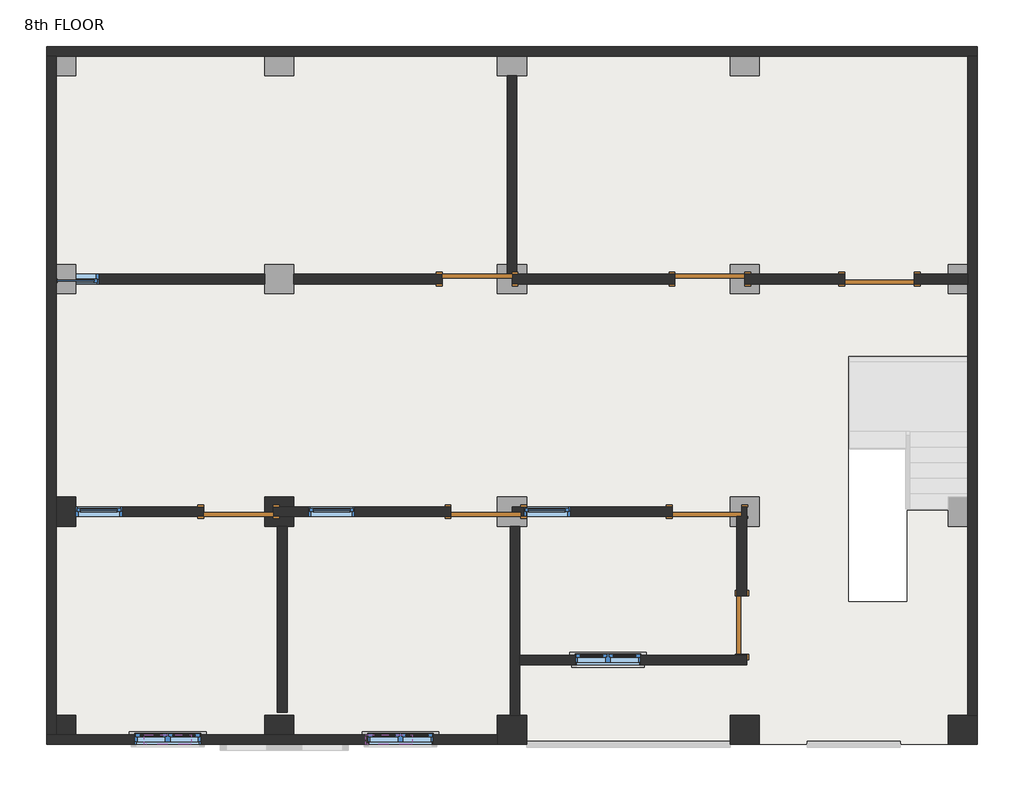
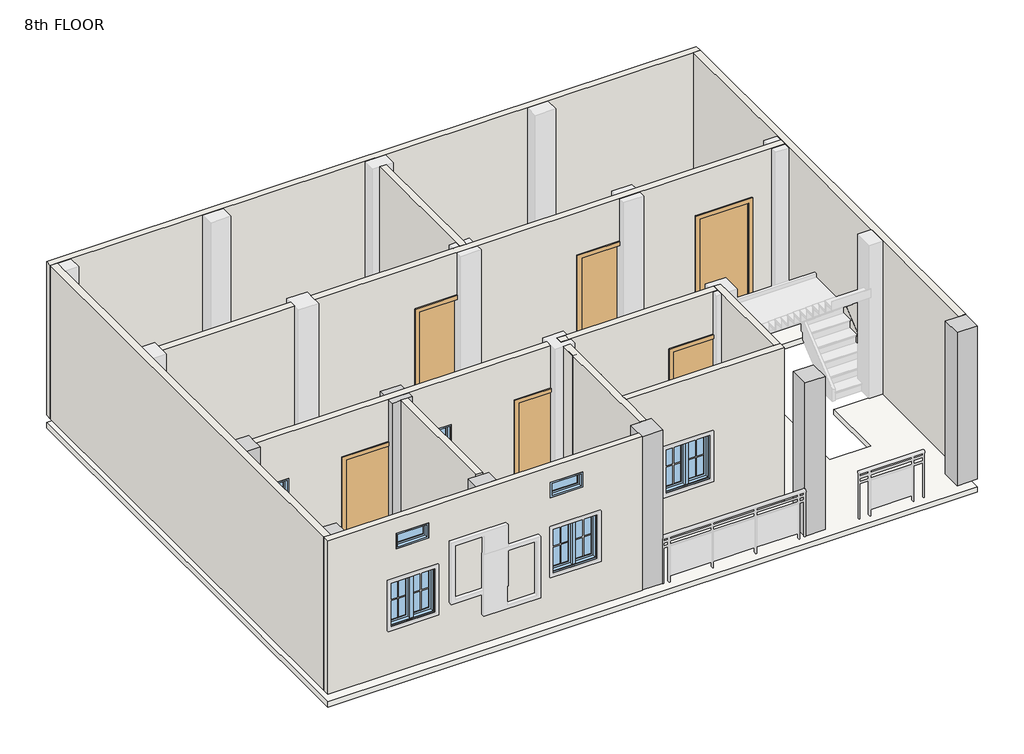
# One storey, part 1 of 2: 15 walls, 9 windows, 7 columns, 7 doors, 1 slab.
"""IFC4 building model written with IfcOpenShell, lengths in millimetres."""

from ifc_helpers import new_model, si_unit, frame, origin, place, context, project, spatial, polyline, outline, extrude, faceted_brep, transform, mapped, element, save
from components import door_e00f436c, door_a1797ceb, window_4c2727af, window_0bf3737e, window_78893e6c, window_0d9958e7

model = new_model("IFC4")

# Units and contexts
model_context = context("Model", 3, world=origin())
ifc_project = project(units=[si_unit("LENGTHUNIT", "METRE", prefix="MILLI")], contexts=[model_context])

# Site, building, storey
site = spatial("IfcSite", under=ifc_project)
building = spatial("IfcBuilding", under=site)
storey = spatial("IfcBuildingStorey", under=building, Name="8th FLOOR", Elevation=24231.6)

# Columns
placement = place(None, origin())
element("IfcColumn", 1, ObjectType="column family : column family", at=placement, inside=storey, context=model_context, shape_type="Brep", body=[
    faceted_brep([(-12576.097125, 2486.2065522, 24236.6), (-12957.097125, 2486.2065522, 24236.6), (-12957.097125, 2867.2065522, 24236.6), (-12576.097125, 2867.2065522, 24236.6), (-12576.097125, 2740.2065522, 24236.6), (-12842.797125, 2740.2065522, 24236.6), (-12842.797125, 2613.2065522, 24236.6), (-12576.097125, 2613.2065522, 24236.6), (-12576.097125, 2486.2065522, 27274.6), (-12576.097125, 2613.2065522, 27274.6), (-12957.097125, 2486.2065522, 27274.6), (-12957.097125, 2613.2065522, 27274.6), (-12957.097125, 2613.2065522, 26365.2), (-12957.097125, 2740.2065522, 26365.2), (-12957.097125, 2740.2065522, 27274.6), (-12957.097125, 2867.2065522, 27274.6), (-12576.097125, 2867.2065522, 27274.6), (-12842.797125, 2613.2065522, 26365.2), (-12842.797125, 2740.2065522, 26365.2), (-12576.097125, 2740.2065522, 27274.6)], [[[0, 1, 2, 3, 4, 5, 6, 7]], [[8, 0, 7, 9]], [[1, 0, 8, 10]], [[2, 1, 10, 11, 12, 13, 14, 15]], [[3, 2, 15, 16]], [[10, 8, 9, 11]], [[6, 17, 12, 11, 9, 7]], [[13, 18, 5, 4, 19, 14]], [[3, 16, 19, 4]], [[16, 15, 14, 19]], [[17, 18, 13, 12]], [[18, 17, 6, 5]]]),
])
element("IfcColumn", 2, ObjectType="column family : column family", at=placement, inside=storey, context=model_context, shape_type="SweptSolid", body=[
    extrude(outline(polyline([(-15433.597125, 2867.2065522), (-15433.597125, 2486.2065522), (-15687.597125, 2486.2065522), (-15687.597125, 2867.2065522), (-15433.597125, 2867.2065522)])), frame((0.0, 0.0, 24236.6), z_axis=(0.0, 0.0, 1.0), x_axis=(1.0, 0.0, 0.0)), (0.0, 0.0, 1.0), 3038.0),
])
element("IfcColumn", 3, ObjectType="column family : column family", at=placement, inside=storey, context=model_context, shape_type="SweptSolid", body=[
    extrude(outline(polyline([(-15433.597125, 9.7065522), (-15433.597125, -244.2934478), (-15687.597125, -244.2934478), (-15687.597125, 9.7065522), (-15433.597125, 9.7065522)])), frame((0.0, 0.0, 24236.6), z_axis=(0.0, 0.0, 1.0), x_axis=(1.0, 0.0, 0.0)), (0.0, 0.0, 1.0), 3038.0),
])
element("IfcColumn", 4, ObjectType="column family : column family", at=placement, inside=storey, context=model_context, shape_type="SweptSolid", body=[
    extrude(outline(polyline([(-3622.597125, 9.7065522), (-3622.597125, -371.2934478), (-4003.597125, -371.2934478), (-4003.597125, 9.7065522), (-3622.597125, 9.7065522)])), frame((0.0, 0.0, 24236.6), z_axis=(0.0, 0.0, 1.0), x_axis=(1.0, 0.0, 0.0)), (0.0, 0.0, 1.0), 3038.0),
])
element("IfcColumn", 5, ObjectType="column family : column family", at=placement, inside=storey, context=model_context, shape_type="SweptSolid", body=[
    extrude(outline(polyline([(-6480.097125, 9.7065522), (-6480.097125, -371.2934478), (-6861.097125, -371.2934478), (-6861.097125, 9.7065522), (-6480.097125, 9.7065522)])), frame((0.0, 0.0, 24236.6), z_axis=(0.0, 0.0, 1.0), x_axis=(1.0, 0.0, 0.0)), (0.0, 0.0, 1.0), 3038.0),
])
element("IfcColumn", 6, ObjectType="column family : column family", at=placement, inside=storey, context=model_context, shape_type="SweptSolid", body=[
    extrude(outline(polyline([(-9528.097125, 9.7065522), (-9528.097125, -371.2934478), (-9909.097125, -371.2934478), (-9909.097125, 9.7065522), (-9528.097125, 9.7065522)])), frame((0.0, 0.0, 24236.6), z_axis=(0.0, 0.0, 1.0), x_axis=(1.0, 0.0, 0.0)), (0.0, 0.0, 1.0), 3038.0),
])
element("IfcColumn", 7, ObjectType="column family : column family", at=placement, inside=storey, context=model_context, shape_type="SweptSolid", body=[
    extrude(outline(polyline([(-12957.097125, 9.7065522), (-12576.097125, 9.7065522), (-12576.097125, -244.2934478), (-12957.097125, -244.2934478), (-12957.097125, 9.7065522)])), frame((0.0, 0.0, 24236.6), z_axis=(0.0, 0.0, 1.0), x_axis=(1.0, 0.0, 0.0)), (0.0, 0.0, 1.0), 3038.0),
])

# Doors
door_shape = door_e00f436c(model_context)
element("IfcDoor", 8, ObjectType="Single-Flush : 30\" x 80\"", at=placement, inside=storey, context=model_context, shape_type="MappedRepresentation", body=[
    mapped(door_shape, transform((-6708.697125, 1190.8065522, 24231.6), x_axis=(0.0, -1.0, 0.0), y_axis=(1.0, 0.0, 0.0), z_axis=(0.0, 0.0, 1.0))),
])
door_2_shape = door_a1797ceb(model_context)
element("IfcDoor", 9, ObjectType="Single-Flush : 36\" x 84\"", at=placement, inside=storey, context=model_context, shape_type="MappedRepresentation", body=[
    mapped(door_2_shape, transform((-10175.797125, 5724.7065522, 24231.6), x_axis=(1.0, 0.0, 0.0), y_axis=(0.0, 1.0, 0.0), z_axis=(0.0, 0.0, 1.0))),
])
element("IfcDoor", 10, ObjectType="Single-Flush : 36\" x 84\"", at=placement, inside=storey, context=model_context, shape_type="MappedRepresentation", body=[
    mapped(door_2_shape, transform((-10061.497125, 2676.7065522, 24231.6), x_axis=(-1.0, 0.0, 0.0), y_axis=(0.0, -1.0, 0.0), z_axis=(0.0, 0.0, 1.0))),
])
element("IfcDoor", 11, ObjectType="Single-Flush : 36\" x 84\"", at=placement, inside=storey, context=model_context, shape_type="MappedRepresentation", body=[
    mapped(door_2_shape, transform((-13299.997125, 2676.7065522, 24231.6), x_axis=(-1.0, 0.0, 0.0), y_axis=(0.0, -1.0, 0.0), z_axis=(0.0, 0.0, 1.0))),
])
element("IfcDoor", 12, ObjectType="Single-Flush : 36\" x 84\"", at=placement, inside=storey, context=model_context, shape_type="MappedRepresentation", body=[
    mapped(door_2_shape, transform((-7127.797125, 5724.7065522, 24231.6), x_axis=(1.0, 0.0, 0.0), y_axis=(0.0, 1.0, 0.0), z_axis=(0.0, 0.0, 1.0))),
])
element("IfcDoor", 13, ObjectType="Single-Flush : 36\" x 84\"", at=placement, inside=storey, context=model_context, shape_type="MappedRepresentation", body=[
    mapped(door_2_shape, transform((-7165.897125, 2676.7065522, 24231.6), x_axis=(-1.0, 0.0, 0.0), y_axis=(0.0, -1.0, 0.0), z_axis=(0.0, 0.0, 1.0))),
])
element("IfcDoor", 14, ObjectType="Single-Flush : 36\" x 84\"", at=placement, inside=storey, context=model_context, shape_type="MappedRepresentation", body=[
    mapped(door_2_shape, transform((-4905.297125, 5724.7065522, 24231.6), x_axis=(-1.0, 0.0, 0.0), y_axis=(0.0, -1.0, 0.0), z_axis=(0.0, 0.0, 1.0))),
])

# Slab
element("IfcSlab", 15, ObjectType="Generic - 4\"", at=placement, inside=storey, context=model_context, shape_type="SweptSolid", body=[
    extrude(outline(polyline([(-3622.597125, 8772.7065522), (-3622.597125, -371.2934478), (-15814.597125, -371.2934478), (-15814.597125, 8772.7065522), (-3622.597125, 8772.7065522)]), holes=[polyline([(-3734.357125, 4711.0719226), (-5310.2646464, 4711.0719226), (-5310.2646464, 1502.3126957), (-4547.7736682, 1502.3126957), (-4547.7736682, 2699.911213), (-3734.357125, 2699.911213), (-3734.357125, 4711.0719226)])]), frame((0.0, 0.0, 23977.6), z_axis=(0.0, 0.0, 1.0), x_axis=(1.0, 0.0, 0.0)), (0.0, 0.0, 1.0), 101.6),
])

# Walls
element("IfcWall", 16, ObjectType="Generic - 5\"", at=placement, inside=storey, context=model_context, shape_type="Brep", body=[
    faceted_brep([(-15814.597125, 8645.7065522, 24231.6), (-15687.597125, 8645.7065522, 24231.6), (-3749.597125, 8645.7065522, 24231.6), (-3622.597125, 8645.7065522, 24231.6), (-3622.597125, 8645.7065522, 27279.6), (-3749.597125, 8645.7065522, 27279.6), (-15687.597125, 8645.7065522, 27279.6), (-15814.597125, 8645.7065522, 27279.6), (-15814.597125, 8772.7065522, 24231.6), (-15814.597125, 8772.7065522, 27279.6), (-3622.597125, 8772.7065522, 27279.6), (-3622.597125, 8772.7065522, 24231.6)], [[[0, 1, 2, 3, 4, 5, 6, 7]], [[8, 9, 10, 11]], [[3, 2, 1, 0, 8, 11]], [[7, 6, 5, 4, 10, 9]], [[4, 3, 11, 10]], [[0, 7, 9, 8]]]),
])
element("IfcWall", 17, ObjectType="Generic - 5\"", at=placement, inside=storey, context=model_context, shape_type="Brep", body=[
    faceted_brep([(-3749.597125, 8645.7065522, 24231.6), (-3749.597125, 5788.2065522, 24231.6), (-3749.597125, 5661.2065522, 24231.6), (-3749.597125, 9.7065522, 24231.6), (-3749.597125, 9.7065522, 27279.6), (-3749.597125, 5661.2065522, 27279.6), (-3749.597125, 5788.2065522, 27279.6), (-3749.597125, 8645.7065522, 27279.6), (-3622.597125, 8645.7065522, 24231.6), (-3622.597125, 8645.7065522, 27279.6), (-3622.597125, 9.7065522, 27279.6), (-3622.597125, 9.7065522, 27274.6), (-3622.597125, 9.7065522, 24236.6), (-3622.597125, 9.7065522, 24231.6)], [[[0, 1, 2, 3, 4, 5, 6, 7]], [[8, 9, 10, 11, 12, 13]], [[3, 2, 1, 0, 8, 13]], [[4, 3, 13, 12, 11, 10]], [[7, 6, 5, 4, 10, 9]], [[0, 7, 9, 8]]]),
])
element("IfcWall", 18, ObjectType="Generic - 5\"", at=placement, inside=storey, context=model_context, shape_type="Brep", body=[
    faceted_brep([(-9909.097125, -244.2934478, 24231.6), (-15687.597125, -244.2934478, 24231.6), (-15814.597125, -244.2934478, 24231.6), (-15814.597125, -244.2934478, 27279.6), (-15687.597125, -244.2934478, 27279.6), (-9909.097125, -244.2934478, 27279.6), (-13795.297125, -244.2934478, 26060.4), (-14658.897125, -244.2934478, 26060.4), (-14658.897125, -244.2934478, 25146.0), (-13795.297125, -244.2934478, 25146.0), (-10747.297125, -244.2934478, 26060.4), (-11610.897125, -244.2934478, 26060.4), (-11610.897125, -244.2934478, 25146.0), (-10747.297125, -244.2934478, 25146.0), (-13922.297125, -244.2934478, 26974.8), (-14531.897125, -244.2934478, 26974.8), (-14531.897125, -244.2934478, 26670.0), (-13922.297125, -244.2934478, 26670.0), (-11026.697125, -244.2934478, 26974.8), (-11636.297125, -244.2934478, 26974.8), (-11636.297125, -244.2934478, 26670.0), (-11026.697125, -244.2934478, 26670.0), (-9909.097125, -371.2934478, 24231.6), (-9909.097125, -371.2934478, 24236.6), (-9909.097125, -371.2934478, 27274.6), (-9909.097125, -371.2934478, 27279.6), (-15814.597125, -371.2934478, 27279.6), (-15814.597125, -371.2934478, 24231.6), (-13795.297125, -371.2934478, 26060.4), (-13795.297125, -371.2934478, 25146.0), (-14658.897125, -371.2934478, 25146.0), (-14658.897125, -371.2934478, 26060.4), (-10747.297125, -371.2934478, 26060.4), (-10747.297125, -371.2934478, 25146.0), (-11610.897125, -371.2934478, 25146.0), (-11610.897125, -371.2934478, 26060.4), (-13922.297125, -371.2934478, 26974.8), (-13922.297125, -371.2934478, 26670.0), (-14531.897125, -371.2934478, 26670.0), (-14531.897125, -371.2934478, 26974.8), (-11026.697125, -371.2934478, 26974.8), (-11026.697125, -371.2934478, 26670.0), (-11636.297125, -371.2934478, 26670.0), (-11636.297125, -371.2934478, 26974.8)], [[[0, 1, 2, 3, 4, 5], [6, 7, 8, 9], [10, 11, 12, 13], [14, 15, 16, 17], [18, 19, 20, 21]], [[22, 23, 24, 25, 26, 27], [28, 29, 30, 31], [32, 33, 34, 35], [36, 37, 38, 39], [40, 41, 42, 43]], [[2, 1, 0, 22, 27]], [[5, 4, 3, 26, 25]], [[0, 5, 25, 24, 23, 22]], [[3, 2, 27, 26]], [[29, 28, 6, 9]], [[30, 29, 9, 8]], [[31, 30, 8, 7]], [[28, 31, 7, 6]], [[33, 32, 10, 13]], [[34, 33, 13, 12]], [[35, 34, 12, 11]], [[32, 35, 11, 10]], [[37, 36, 14, 17]], [[38, 37, 17, 16]], [[39, 38, 16, 15]], [[36, 39, 15, 14]], [[41, 40, 18, 21]], [[42, 41, 21, 20]], [[43, 42, 20, 19]], [[40, 43, 19, 18]]]),
])
element("IfcWall", 19, ObjectType="Generic - 5\"", at=placement, inside=storey, context=model_context, shape_type="Brep", body=[
    faceted_brep([(-15687.597125, -244.2934478, 24231.6), (-15687.597125, 8645.7065522, 24231.6), (-15687.597125, 8645.7065522, 24236.6), (-15687.597125, 8645.7065522, 27274.6), (-15687.597125, 8645.7065522, 27279.6), (-15687.597125, -244.2934478, 27279.6), (-15687.597125, -244.2934478, 27274.6), (-15687.597125, -244.2934478, 24236.6), (-15814.597125, -244.2934478, 24231.6), (-15814.597125, -244.2934478, 27279.6), (-15814.597125, 8645.7065522, 27279.6), (-15814.597125, 8645.7065522, 24231.6)], [[[0, 1, 2, 3, 4, 5, 6, 7]], [[8, 9, 10, 11]], [[1, 0, 8, 11]], [[5, 4, 10, 9]], [[4, 3, 2, 1, 11, 10]], [[0, 7, 6, 5, 9, 8]]]),
])
element("IfcWall", 20, ObjectType="Generic - 5\"", at=placement, inside=storey, context=model_context, shape_type="SweptSolid", body=[
    extrude(outline(polyline([(24231.6, -15433.597125), (24231.6, -12957.097125), (27279.6, -12957.097125), (27279.6, -15433.597125), (26365.2, -15433.597125), (26365.2, -15128.797125), (24536.4, -15128.797125), (24536.4, -15433.597125), (24231.6, -15433.597125)])), frame((0.0, 5661.2065522, 0.0), z_axis=(0.0, 1.0, 0.0), x_axis=(0.0, 0.0, 1.0)), (0.0, 0.0, 1.0), 127.0),
])
element("IfcWall", 21, ObjectType="Generic - 5\"", at=placement, inside=storey, context=model_context, shape_type="Brep", body=[
    faceted_brep([(-9782.097125, 8391.7065522, 24231.6), (-9782.097125, 5788.2065522, 24231.6), (-9782.097125, 5788.2065522, 24236.6), (-9782.097125, 5788.2065522, 26365.2), (-9782.097125, 5788.2065522, 27274.6), (-9782.097125, 5788.2065522, 27279.6), (-9782.097125, 8391.7065522, 27279.6), (-9655.097125, 8391.7065522, 24231.6), (-9655.097125, 8391.7065522, 27279.6), (-9655.097125, 5788.2065522, 27279.6), (-9655.097125, 5788.2065522, 27274.6), (-9655.097125, 5788.2065522, 24236.6), (-9655.097125, 5788.2065522, 24231.6), (-9718.597125, 5788.2065522, 24231.6)], [[[0, 1, 2, 3, 4, 5, 6]], [[7, 8, 9, 10, 11, 12]], [[1, 0, 7, 12, 13]], [[6, 5, 9, 8]], [[0, 6, 8, 7]], [[5, 4, 3, 2, 1, 13, 12, 11, 10, 9]]]),
])
element("IfcWall", 22, ObjectType="Generic - 5\"", at=placement, inside=storey, context=model_context, shape_type="Brep", body=[
    faceted_brep([(-6670.597125, 5661.2065522, 24231.6), (-5362.497125, 5661.2065522, 24231.6), (-5362.497125, 5661.2065522, 26365.2), (-4448.097125, 5661.2065522, 26365.2), (-4448.097125, 5661.2065522, 24231.6), (-3749.597125, 5661.2065522, 24231.6), (-3749.597125, 5661.2065522, 24236.6), (-3749.597125, 5661.2065522, 27274.6), (-3749.597125, 5661.2065522, 27279.6), (-12576.097125, 5661.2065522, 27279.6), (-12576.097125, 5661.2065522, 24231.6), (-10632.997125, 5661.2065522, 24231.6), (-10632.997125, 5661.2065522, 26365.2), (-9909.097125, 5661.2065522, 26365.2), (-9718.597125, 5661.2065522, 26365.2), (-9718.597125, 5661.2065522, 24236.6), (-9718.597125, 5661.2065522, 24231.6), (-7584.997125, 5661.2065522, 24231.6), (-7584.997125, 5661.2065522, 26365.2), (-6861.097125, 5661.2065522, 26365.2), (-6670.597125, 5661.2065522, 26365.2), (-6670.597125, 5661.2065522, 24236.6), (-5362.497125, 5788.2065522, 26365.2), (-5362.497125, 5788.2065522, 24231.6), (-6670.597125, 5788.2065522, 24231.6), (-6670.597125, 5788.2065522, 24236.6), (-6670.597125, 5788.2065522, 26365.2), (-6861.097125, 5788.2065522, 26365.2), (-7584.997125, 5788.2065522, 26365.2), (-7584.997125, 5788.2065522, 24231.6), (-9655.097125, 5788.2065522, 24231.6), (-9718.597125, 5788.2065522, 24231.6), (-9718.597125, 5788.2065522, 24236.6), (-9718.597125, 5788.2065522, 26365.2), (-9782.097125, 5788.2065522, 26365.2), (-9909.097125, 5788.2065522, 26365.2), (-10632.997125, 5788.2065522, 26365.2), (-10632.997125, 5788.2065522, 24231.6), (-12576.097125, 5788.2065522, 24231.6), (-12576.097125, 5788.2065522, 27279.6), (-9782.097125, 5788.2065522, 27279.6), (-9655.097125, 5788.2065522, 27279.6), (-3749.597125, 5788.2065522, 27279.6), (-3749.597125, 5788.2065522, 27274.6), (-3749.597125, 5788.2065522, 24236.6), (-3749.597125, 5788.2065522, 24231.6), (-4448.097125, 5788.2065522, 24231.6), (-4448.097125, 5788.2065522, 26365.2)], [[[0, 1, 2, 3, 4, 5, 6, 7, 8, 9, 10, 11, 12, 13, 14, 15, 16, 17, 18, 19, 20, 21]], [[22, 23, 24, 25, 26, 27, 28, 29, 30, 31, 32, 33, 34, 35, 36, 37, 38, 39, 40, 41, 42, 43, 44, 45, 46, 47]], [[11, 10, 38, 37]], [[17, 16, 31, 30, 29]], [[46, 45, 5, 4]], [[24, 23, 1, 0]], [[9, 8, 42, 41, 40, 39]], [[10, 9, 39, 38]], [[8, 7, 6, 5, 45, 44, 43, 42]], [[33, 32, 31, 16, 15, 14]], [[36, 35, 34, 33, 14, 13, 12]], [[37, 36, 12, 11]], [[26, 25, 24, 0, 21, 20]], [[28, 27, 26, 20, 19, 18]], [[29, 28, 18, 17]], [[2, 1, 23, 22]], [[3, 2, 22, 47]], [[4, 3, 47, 46]]]),
])
element("IfcWall", 23, ObjectType="Generic - 5\"", at=placement, inside=storey, context=model_context, shape_type="Brep", body=[
    faceted_brep([(-14823.997125, 2613.2065522, 24536.4), (-15433.597125, 2613.2065522, 24536.4), (-15433.597125, 2613.2065522, 24231.6), (-13757.197125, 2613.2065522, 24231.6), (-13757.197125, 2613.2065522, 26365.2), (-12957.097125, 2613.2065522, 26365.2), (-12842.797125, 2613.2065522, 26365.2), (-12842.797125, 2613.2065522, 24236.6), (-12842.797125, 2613.2065522, 24231.6), (-10518.697125, 2613.2065522, 24231.6), (-10518.697125, 2613.2065522, 26365.2), (-9909.097125, 2613.2065522, 26365.2), (-9909.097125, 2613.2065522, 27279.6), (-15433.597125, 2613.2065522, 27279.6), (-15433.597125, 2613.2065522, 26365.2), (-14823.997125, 2613.2065522, 26365.2), (-12385.597125, 2613.2065522, 26365.2), (-11775.997125, 2613.2065522, 26365.2), (-11775.997125, 2613.2065522, 24536.4), (-12385.597125, 2613.2065522, 24536.4), (-15433.597125, 2740.2065522, 24231.6), (-15433.597125, 2740.2065522, 24536.4), (-14823.997125, 2740.2065522, 24536.4), (-14823.997125, 2740.2065522, 26365.2), (-15433.597125, 2740.2065522, 26365.2), (-15433.597125, 2740.2065522, 27279.6), (-9909.097125, 2740.2065522, 27279.6), (-9909.097125, 2740.2065522, 26365.2), (-10518.697125, 2740.2065522, 26365.2), (-10518.697125, 2740.2065522, 24231.6), (-12842.797125, 2740.2065522, 24231.6), (-12842.797125, 2740.2065522, 24236.6), (-12842.797125, 2740.2065522, 26365.2), (-12957.097125, 2740.2065522, 26365.2), (-13757.197125, 2740.2065522, 26365.2), (-13757.197125, 2740.2065522, 24231.6), (-12385.597125, 2740.2065522, 26365.2), (-12385.597125, 2740.2065522, 24536.4), (-11775.997125, 2740.2065522, 24536.4), (-11775.997125, 2740.2065522, 26365.2)], [[[0, 1, 2, 3, 4, 5, 6, 7, 8, 9, 10, 11, 12, 13, 14, 15], [16, 17, 18, 19]], [[20, 21, 22, 23, 24, 25, 26, 27, 28, 29, 30, 31, 32, 33, 34, 35], [36, 37, 38, 39]], [[30, 29, 9, 8]], [[20, 35, 3, 2]], [[26, 12, 11, 27]], [[13, 12, 26, 25]], [[14, 13, 25, 24]], [[2, 1, 21, 20]], [[28, 10, 9, 29]], [[10, 28, 27, 11]], [[4, 3, 35, 34]], [[6, 5, 4, 34, 33, 32]], [[8, 7, 6, 32, 31, 30]], [[22, 21, 1, 0]], [[23, 22, 0, 15]], [[24, 23, 15, 14]], [[37, 36, 16, 19]], [[38, 37, 19, 18]], [[39, 38, 18, 17]], [[36, 39, 17, 16]]]),
])
element("IfcWall", 24, ObjectType="Generic - 5\"", at=placement, inside=storey, context=model_context, shape_type="Brep", body=[
    faceted_brep([(-9616.997125, 9.7065522, 24231.6), (-9616.997125, 670.1065522, 24231.6), (-9616.997125, 797.1065522, 24231.6), (-9616.997125, 2486.2065522, 24231.6), (-9616.997125, 2486.2065522, 27279.6), (-9616.997125, 797.1065522, 27279.6), (-9616.997125, 670.1065522, 27279.6), (-9616.997125, 9.7065522, 27279.6), (-9743.997125, 9.7065522, 24231.6), (-9743.997125, 9.7065522, 27279.6), (-9743.997125, 2486.2065522, 27279.6), (-9743.997125, 2486.2065522, 24231.6)], [[[0, 1, 2, 3, 4, 5, 6, 7]], [[8, 9, 10, 11]], [[3, 2, 1, 0, 8, 11]], [[4, 3, 11, 10]], [[7, 6, 5, 4, 10, 9]], [[0, 7, 9, 8]]]),
])
element("IfcWall", 25, ObjectType="Generic - 5\"", at=placement, inside=storey, context=model_context, shape_type="SweptSolid", body=[
    extrude(outline(polyline([(-9743.997125, 2181.4065522), (-9743.997125, 2486.2065522), (-9616.997125, 2486.2065522), (-9616.997125, 2181.4065522), (-9743.997125, 2181.4065522)])), frame((0.0, 0.0, 24231.6), z_axis=(0.0, 0.0, 1.0), x_axis=(1.0, 0.0, 0.0)), (0.0, 0.0, 1.0), 3048.0),
])
element("IfcWall", 26, ObjectType="Generic - 5\"", at=placement, inside=storey, context=model_context, shape_type="Brep", body=[
    faceted_brep([(-6772.197125, 2613.2065522, 27279.6), (-9718.597125, 2613.2065522, 27279.6), (-9718.597125, 2613.2065522, 27274.6), (-9718.597125, 2613.2065522, 24236.6), (-9718.597125, 2613.2065522, 24231.6), (-7623.097125, 2613.2065522, 24231.6), (-7623.097125, 2613.2065522, 26365.2), (-6861.097125, 2613.2065522, 26365.2), (-6772.197125, 2613.2065522, 26365.2), (-6772.197125, 2613.2065522, 27274.6), (-9566.197125, 2613.2065522, 26365.2), (-9528.097125, 2613.2065522, 26365.2), (-8956.597125, 2613.2065522, 26365.2), (-8956.597125, 2613.2065522, 24536.4), (-9528.097125, 2613.2065522, 24536.4), (-9566.197125, 2613.2065522, 24536.4), (-9718.597125, 2740.2065522, 27279.6), (-6772.197125, 2740.2065522, 27279.6), (-6772.197125, 2740.2065522, 26365.2), (-6861.097125, 2740.2065522, 26365.2), (-7623.097125, 2740.2065522, 26365.2), (-7623.097125, 2740.2065522, 24231.6), (-9718.597125, 2740.2065522, 24231.6), (-9718.597125, 2740.2065522, 24236.6), (-9718.597125, 2740.2065522, 27274.6), (-9566.197125, 2740.2065522, 26365.2), (-9566.197125, 2740.2065522, 24536.4), (-9528.097125, 2740.2065522, 24536.4), (-8956.597125, 2740.2065522, 24536.4), (-8956.597125, 2740.2065522, 26365.2), (-9528.097125, 2740.2065522, 26365.2)], [[[0, 1, 2, 3, 4, 5, 6, 7, 8, 9], [10, 11, 12, 13, 14, 15]], [[16, 17, 18, 19, 20, 21, 22, 23, 24], [25, 26, 27, 28, 29, 30]], [[4, 22, 21, 5]], [[1, 0, 17, 16]], [[4, 3, 2, 1, 16, 24, 23, 22]], [[26, 25, 10, 15]], [[28, 27, 26, 15, 14, 13]], [[29, 28, 13, 12]], [[25, 30, 29, 12, 11, 10]], [[20, 6, 5, 21]], [[6, 20, 19, 18, 8, 7]], [[17, 0, 9, 8, 18]]]),
])
element("IfcWall", 27, ObjectType="Generic - 5\"", at=placement, inside=storey, context=model_context, shape_type="Brep", body=[
    faceted_brep([(-6645.197125, 797.1065522, 24231.6), (-6645.197125, 809.8065522, 24231.6), (-6645.197125, 809.8065522, 26263.6), (-6645.197125, 1571.8065522, 26263.6), (-6645.197125, 1571.8065522, 24231.6), (-6645.197125, 2740.2065522, 24231.6), (-6645.197125, 2740.2065522, 24236.6), (-6645.197125, 2740.2065522, 27274.6), (-6645.197125, 2740.2065522, 27279.6), (-6645.197125, 797.1065522, 27279.6), (-6772.197125, 809.8065522, 26263.6), (-6772.197125, 809.8065522, 24231.6), (-6772.197125, 797.1065522, 24231.6), (-6772.197125, 797.1065522, 27279.6), (-6772.197125, 2613.2065522, 27279.6), (-6772.197125, 2740.2065522, 27279.6), (-6772.197125, 2740.2065522, 26365.2), (-6772.197125, 2613.2065522, 26365.2), (-6772.197125, 2613.2065522, 24236.6), (-6772.197125, 2613.2065522, 24231.6), (-6772.197125, 1571.8065522, 24231.6), (-6772.197125, 1571.8065522, 26263.6), (-6708.697125, 2613.2065522, 24231.6), (-6708.697125, 2740.2065522, 24231.6), (-6708.697125, 2613.2065522, 26365.2), (-6708.697125, 2613.2065522, 24236.6), (-6708.697125, 2740.2065522, 26365.2), (-6708.697125, 2740.2065522, 24236.6)], [[[0, 1, 2, 3, 4, 5, 6, 7, 8, 9]], [[10, 11, 12, 13, 14, 15, 16, 17, 18, 19, 20, 21]], [[20, 19, 22, 23, 5, 4]], [[12, 11, 1, 0]], [[9, 8, 15, 14, 13]], [[24, 25, 22, 19, 18, 17]], [[26, 24, 17, 16]], [[22, 25, 24, 26, 27, 23]], [[8, 7, 6, 5, 23, 27, 26, 16, 15]], [[0, 9, 13, 12]], [[2, 1, 11, 10]], [[3, 2, 10, 21]], [[4, 3, 21, 20]]]),
])
element("IfcWall", 28, ObjectType="Generic - 5\"", at=placement, inside=storey, context=model_context, shape_type="Brep", body=[
    faceted_brep([(-9718.597125, 2613.2065522, 24231.6), (-9566.197125, 2613.2065522, 24231.6), (-9566.197125, 2613.2065522, 24536.4), (-9566.197125, 2613.2065522, 26365.2), (-9566.197125, 2613.2065522, 27279.6), (-9718.597125, 2613.2065522, 27279.6), (-9718.597125, 2613.2065522, 27274.6), (-9718.597125, 2613.2065522, 24236.6), (-9718.597125, 2740.2065522, 24231.6), (-9718.597125, 2740.2065522, 24236.6), (-9718.597125, 2740.2065522, 27274.6), (-9718.597125, 2740.2065522, 27279.6), (-9566.197125, 2740.2065522, 27279.6), (-9566.197125, 2740.2065522, 26365.2), (-9566.197125, 2740.2065522, 24536.4), (-9566.197125, 2740.2065522, 24231.6)], [[[0, 1, 2, 3, 4, 5, 6, 7]], [[8, 9, 10, 11, 12, 13, 14, 15]], [[1, 0, 8, 15]], [[4, 3, 2, 1, 15, 14, 13, 12]], [[5, 4, 12, 11]], [[0, 7, 6, 5, 11, 10, 9, 8]]]),
])
element("IfcWall", 29, ObjectType="Generic - 5\"", at=placement, inside=storey, context=model_context, shape_type="SweptSolid", body=[
    extrude(outline(polyline([(-12791.997125, 47.8065522), (-12791.997125, 2486.2065522), (-12664.997125, 2486.2065522), (-12664.997125, 47.8065522), (-12791.997125, 47.8065522)])), frame((0.0, 0.0, 24231.6), z_axis=(0.0, 0.0, 1.0), x_axis=(1.0, 0.0, 0.0)), (0.0, 0.0, 1.0), 3048.0),
])
element("IfcWall", 30, ObjectType="Generic - 5\"", at=placement, inside=storey, context=model_context, shape_type="Brep", body=[
    faceted_brep([(-9616.997125, 670.1065522, 24231.6), (-6645.197125, 670.1065522, 24231.6), (-6645.197125, 670.1065522, 27279.6), (-9616.997125, 670.1065522, 27279.6), (-8029.497125, 670.1065522, 26060.4), (-8029.497125, 670.1065522, 25146.0), (-8893.097125, 670.1065522, 25146.0), (-8893.097125, 670.1065522, 26060.4), (-9616.997125, 797.1065522, 24231.6), (-9616.997125, 797.1065522, 27279.6), (-6772.197125, 797.1065522, 27279.6), (-6645.197125, 797.1065522, 27279.6), (-6645.197125, 797.1065522, 24231.6), (-6772.197125, 797.1065522, 24231.6), (-8029.497125, 797.1065522, 26060.4), (-8893.097125, 797.1065522, 26060.4), (-8893.097125, 797.1065522, 25146.0), (-8029.497125, 797.1065522, 25146.0)], [[[0, 1, 2, 3], [4, 5, 6, 7]], [[8, 9, 10, 11, 12, 13], [14, 15, 16, 17]], [[1, 0, 8, 13, 12]], [[3, 2, 11, 10, 9]], [[0, 3, 9, 8]], [[2, 1, 12, 11]], [[5, 4, 14, 17]], [[6, 5, 17, 16]], [[7, 6, 16, 15]], [[4, 7, 15, 14]]]),
])

# Windows
window_shape = window_4c2727af(model_context)
element("IfcWindow", 31, ObjectType="Fixed : 24\" x 12\"", at=placement, inside=storey, context=model_context, shape_type="MappedRepresentation", body=[
    mapped(window_shape, transform((-14188.997125, -307.7934478, 25755.6), x_axis=(1.0, 0.0, 0.0), y_axis=(0.0, 1.0, 0.0), z_axis=(0.0, 0.0, 1.0))),
])
element("IfcWindow", 32, ObjectType="Fixed : 24\" x 12\"", at=placement, inside=storey, context=model_context, shape_type="MappedRepresentation", body=[
    mapped(window_shape, transform((-11293.397125, -307.7934478, 25755.6), x_axis=(1.0, 0.0, 0.0), y_axis=(0.0, 1.0, 0.0), z_axis=(0.0, 0.0, 1.0))),
])
window_2_shape = window_0bf3737e(model_context)
element("IfcWindow", 33, ObjectType="Fixed : 24\" x 72\"", at=placement, inside=storey, context=model_context, shape_type="MappedRepresentation", body=[
    mapped(window_2_shape, transform((-15471.697125, 5724.7065522, 24231.6), x_axis=(-1.0, 0.0, 0.0), y_axis=(0.0, -1.0, 0.0), z_axis=(0.0, 0.0, 1.0))),
])
window_3_shape = window_78893e6c(model_context)
element("IfcWindow", 34, ObjectType="Fixed : 24\" x 72\"", at=placement, inside=storey, context=model_context, shape_type="MappedRepresentation", body=[
    mapped(window_3_shape, transform((-15166.897125, 2676.7065522, 24231.6), x_axis=(-1.0, 0.0, 0.0), y_axis=(0.0, -1.0, 0.0), z_axis=(0.0, 0.0, 1.0))),
])
element("IfcWindow", 35, ObjectType="Fixed : 24\" x 72\"", at=placement, inside=storey, context=model_context, shape_type="MappedRepresentation", body=[
    mapped(window_3_shape, transform((-12118.897125, 2676.7065522, 24231.6), x_axis=(-1.0, 0.0, 0.0), y_axis=(0.0, -1.0, 0.0), z_axis=(0.0, 0.0, 1.0))),
])
element("IfcWindow", 36, ObjectType="Fixed : 24\" x 72\"", at=placement, inside=storey, context=model_context, shape_type="MappedRepresentation", body=[
    mapped(window_3_shape, transform((-9299.497125, 2676.7065522, 24231.6), x_axis=(-1.0, 0.0, 0.0), y_axis=(0.0, -1.0, 0.0), z_axis=(0.0, 0.0, 1.0))),
])
window_4_shape = window_0d9958e7(model_context)
element("IfcWindow", 37, ObjectType="Window-Casement-Double : 34\" x 36\"", at=placement, inside=storey, context=model_context, shape_type="MappedRepresentation", body=[
    mapped(window_4_shape, transform((-14227.097125, -307.7934478, 24231.6), x_axis=(1.0, 0.0, 0.0), y_axis=(0.0, 1.0, 0.0), z_axis=(0.0, 0.0, 1.0))),
])
element("IfcWindow", 38, ObjectType="Window-Casement-Double : 34\" x 36\"", at=placement, inside=storey, context=model_context, shape_type="MappedRepresentation", body=[
    mapped(window_4_shape, transform((-11179.097125, -307.7934478, 24231.6), x_axis=(1.0, 0.0, 0.0), y_axis=(0.0, 1.0, 0.0), z_axis=(0.0, 0.0, 1.0))),
])
element("IfcWindow", 39, ObjectType="Window-Casement-Double : 34\" x 36\"", at=placement, inside=storey, context=model_context, shape_type="MappedRepresentation", body=[
    mapped(window_4_shape, transform((-8461.297125, 733.6065522, 24231.6), x_axis=(1.0, 0.0, 0.0), y_axis=(0.0, 1.0, 0.0), z_axis=(0.0, 0.0, 1.0))),
])

save(model, "model.ifc")

# Revit data of these elements
# Type "column family : column family"
#   w2 [instance default] = 0' - 9.88189"
#   w1 [instance default] = 0' - 9.01575"
#   Depth = 1' - 11.62205"
#   Width = 1' - 11.62205"
# Type "Single-Flush : 30\" x 80\""
#   Type Mark = "5"
#   Construction Type Id = "MDOOR"
#   Assembly Code = "C1020"
#   Analytic Construction = "Metal"
#   Thickness = 0' - 2"
#   Heat Transfer Coefficient (U) = 0.651978 BTU/(h·ft²·°F)
#   Height = 6' - 8"
#   Trim Projection Ext = 0' - 1"
#   Trim Projection Int = 0' - 1"
#   Trim Width = 0' - 3"
#   Width = 2' - 6"
#   Define Thermal Properties by = 1
#   Define Thermal Properties by = 1
#   Door Material = Door - Panel
#   Frame Material = Door - Frame
#   Visual Light Transmittance = 0
#   Solar Heat Gain Coefficient = 0
#   Function = (empty or 0)
#   Wall Closure = (empty or 0)
# Type "Single-Flush : 36\" x 84\""
#   Type Mark = "1"
#   Construction Type Id = "MDOOR"
#   Assembly Code = "C1020"
#   Analytic Construction = "Metal"
#   Thickness = 0' - 2"
#   Heat Transfer Coefficient (U) = 0.651978 BTU/(h·ft²·°F)
#   Height = 7' - 0"
#   Trim Projection Ext = 0' - 1"
#   Trim Projection Int = 0' - 1"
#   Trim Width = 0' - 3"
#   Width = 3' - 0"
#   Define Thermal Properties by = 1
#   Define Thermal Properties by = 1
#   Door Material = Door - Panel
#   Frame Material = Door - Frame
#   Visual Light Transmittance = 0
#   Solar Heat Gain Coefficient = 0
#   Function = (empty or 0)
#   Wall Closure = (empty or 0)
# Type "Generic - 4\""
#   Assembly Code = "B1010"
#   Function = 0
#   Layers, outside or top first: 0' - 4" no material (function 1)
# Type "Generic - 5\""
#   Assembly Code = "B2010"
#   Layers, outside or top first: 0' - 5" no material (function 1)
# Type "Fixed : 24\" x 12\""
#   Type Mark = "4"
#   Construction Type Id = "GSP4R"
#   Assembly Code = "B2020100"
#   Analytic Construction = "1/8 in Pilkington single glazing"
#   Visual Light Transmittance = 0.9
#   Solar Heat Gain Coefficient = 0.78
#   Heat Transfer Coefficient (U) = 0.6496 BTU/(h·ft²·°F)
#   Height = 1' - 0"
#   Default Sill Height = 3' - 0"
#   Width = 2' - 0"
#   Window Inset = 0' - 0 3/4"
#   Define Thermal Properties by = 1
#   Define Thermal Properties by = 1
#   Glass Pane Material = Glass
#   Sash Material = Sash
#   Wall Closure = (empty or 0)
# Type "Fixed : 24\" x 72\""
#   Type Mark = "7"
#   Construction Type Id = "GSP4R"
#   Assembly Code = "B2020100"
#   Analytic Construction = "1/8 in Pilkington single glazing"
#   Visual Light Transmittance = 0.9
#   Solar Heat Gain Coefficient = 0.78
#   Heat Transfer Coefficient (U) = 0.6496 BTU/(h·ft²·°F)
#   Height = 6' - 0"
#   Default Sill Height = 1' - 0"
#   Width = 2' - 0"
#   Window Inset = 0' - 0 3/4"
#   Define Thermal Properties by = 1
#   Define Thermal Properties by = 1
#   Glass Pane Material = Glass
#   Sash Material = Sash
#   Wall Closure = (empty or 0)
# Type "Window-Casement-Double : 34\" x 36\""
#   Type Mark = "14"
#   Fire Rating = "0.5h"
#   Assembly Code = "B2020100"
#   Analytic Construction = "Double glazing - domestic"
#   Frame Extension [instance default] = 0' - 0 1/4"
#   Window Inset [instance default] = 0' - 0"
#   Wall Thickness [instance default] = 0' - 6"
#   Interior Wall Closure [instance default] = 0' - 2 1/4"
#   Half Width = 1' - 5"
#   Visual Light Transmittance = 0.81
#   Thermal Resistance (R) = 1.8146 (h·ft²·°F)/BTU
#   Solar Heat Gain Coefficient = 0.76
#   Rough Width = 2' - 10 1/2"
#   Rough Height = 3' - 0 1/2"
#   Height = 3' - 0"
#   Heat Transfer Coefficient (U) = 0.5511 BTU/(h·ft²·°F)
#   Exterior Wall Closure [instance default] = 0' - 1 1/4"
#   Extension Jamb [instance default] = 0' - 2 1/4"
#   Default Sill Height = 3' - 0"
#   Width = 2' - 10"
#   Define Thermal Properties by = 0
#   Muntin Visibility = yes
#   Interior Trim Visibility [instance default] = yes
#   Exterior Trim Visibility [instance default] = yes
#   Extension Jamb Visibility [instance default] = yes
#   Interior Trim Material = Wood - Stained
#   Muntin Pattern = Muntin Pattern_2x2 : Muntin Pattern_2x2
#   Interior Trim = Trim-Window-Interior-Flat : Picture Frame
#   Interior Frame Material = Wood - Stained
#   Glass Panel Material = Glass
#   Exterior Trim Material = Clad - White
#   Exterior Trim = Trim-Window-Exterior-Flat : with Sill
#   Exterior Frame Material = Clad - White
#   Wall Closure = (empty or 0)
# Element 1 (IfcColumn, "column family : column family")
#   w2 = 1' - 3"
#   w1 = 1' - 3"
#   Phase Created = New Construction
#   Materials on its faces: "Default Wall", "inside wall"
# Element 2 (IfcColumn, "column family : column family")
#   w2 = 1' - 3"
#   w1 = 0' - 10"
#   Phase Created = New Construction
#   Materials on its faces: "inside wall", "Default Wall"
# Elements 3, 7 (IfcColumn, "column family : column family")
#   w2 = 1' - 3"
#   w1 = 1' - 3"
#   Phase Created = New Construction
#   Materials on its faces: "Default Wall"
# Element 4 (IfcColumn, "column family : column family")
#   w2 = 1' - 3"
#   w1 = 1' - 3"
#   Phase Created = New Construction
#   Materials on its faces: "Clad - White", "Default Wall"
# Element 5 (IfcColumn, "column family : column family")
#   w2 = 1' - 3"
#   w1 = 1' - 3"
#   Phase Created = New Construction
#   Materials on its faces: "out side wall"
# Element 6 (IfcColumn, "column family : column family")
#   w2 = 1' - 3"
#   w1 = 1' - 3"
#   Phase Created = New Construction
#   Materials on its faces: "out side wall", "Default Wall"
# Element 8 (IfcDoor, "Single-Flush : 30\" x 80\"")
#   Phase Created = New Construction
#   Materials on its faces: "Door - Frame", "Door - Panel"
# Elements 9, 10, 11, 12, 13, 14 (IfcDoor, "Single-Flush : 36\" x 84\"")
#   Phase Created = New Construction
#   Materials on its faces: "Door - Frame", "Door - Panel"
# Element 15 (IfcSlab, "Generic - 4\"")
#   Height Offset From Level = -0' - 6"
#   Phase Created = New Construction
#   Materials on its faces: "Default Floor", "Clad - White", "floor"
# Element 16 (IfcWall, "Generic - 5\"")
#   Top Offset = 0' - 0"
#   Base Offset = 0' - 0"
#   wall height = 10' - 0"
#   Phase Created = New Construction
#   Base Constraint = 8th FLOOR
#   Top Constraint = 9th FLOOR
#   Materials on its faces: "Default Wall", "Clad - White"
# Element 17 (IfcWall, "Generic - 5\"")
#   Top Offset = 0' - 0"
#   Base Offset = 0' - 0"
#   wall height = 10' - 0"
#   Phase Created = New Construction
#   Base Constraint = 8th FLOOR
#   Top Constraint = 9th FLOOR
#   Materials on its faces: "Default Wall", "grey", "Clad - White"
# Element 18 (IfcWall, "Generic - 5\"")
#   Top Offset = 0' - 0"
#   Base Offset = 0' - 0"
#   wall height = 10' - 0"
#   Phase Created = New Construction
#   Base Constraint = 8th FLOOR
#   Top Constraint = 9th FLOOR
#   Materials on its faces: "Default Wall", "out side wall", "Clad - White"
# Element 19 (IfcWall, "Generic - 5\"")
#   Top Offset = 0' - 0"
#   Base Offset = 0' - 0"
#   wall height = 10' - 0"
#   Phase Created = New Construction
#   Base Constraint = 8th FLOOR
#   Top Constraint = 9th FLOOR
#   Materials on its faces: "Default Wall", "inside wall", "Clad - White"
# Elements 20, 23, 26, 27 (IfcWall, "Generic - 5\"")
#   Top Offset = 0' - 0"
#   Base Offset = 0' - 0"
#   wall height = 10' - 0"
#   Phase Created = New Construction
#   Base Constraint = 8th FLOOR
#   Top Constraint = 9th FLOOR
#   Materials on its faces: "Default Wall", "inside wall"
# Elements 21, 25, 28, 29 (IfcWall, "Generic - 5\"")
#   Top Offset = 0' - 0"
#   Base Offset = 0' - 0"
#   wall height = 10' - 0"
#   Phase Created = New Construction
#   Base Constraint = 8th FLOOR
#   Top Constraint = 9th FLOOR
#   Materials on its faces: "Default Wall"
# Elements 22, 24 (IfcWall, "Generic - 5\"")
#   Top Offset = 0' - 0"
#   Base Offset = 0' - 0"
#   wall height = 10' - 0"
#   Phase Created = New Construction
#   Base Constraint = 8th FLOOR
#   Top Constraint = 9th FLOOR
#   Materials on its faces: "Default Wall", "grey"
# Element 30 (IfcWall, "Generic - 5\"")
#   Top Offset = 0' - 0"
#   Base Offset = 0' - 0"
#   wall height = 10' - 0"
#   Phase Created = New Construction
#   Base Constraint = 8th FLOOR
#   Top Constraint = 9th FLOOR
#   Materials on its faces: "Default Wall", "grey", "inside wall"
# Element 31 (IfcWindow, "Fixed : 24\" x 12\"")
#   Mark = "79"
#   Phase Created = New Construction
#   Materials on its faces: "Sash", "Glass"
# Element 32 (IfcWindow, "Fixed : 24\" x 12\"")
#   Mark = "80"
#   Phase Created = New Construction
#   Materials on its faces: "Sash", "Glass"
# Element 33 (IfcWindow, "Fixed : 24\" x 72\"")
#   Mark = "73"
#   Phase Created = New Construction
#   Materials on its faces: "Sash", "Glass"
# Element 34 (IfcWindow, "Fixed : 24\" x 72\"")
#   Mark = "74"
#   Phase Created = New Construction
#   Materials on its faces: "Sash", "Glass"
# Element 35 (IfcWindow, "Fixed : 24\" x 72\"")
#   Mark = "75"
#   Phase Created = New Construction
#   Materials on its faces: "Sash", "Glass"
# Element 36 (IfcWindow, "Fixed : 24\" x 72\"")
#   Mark = "76"
#   Phase Created = New Construction
#   Materials on its faces: "Sash", "Glass"
# Element 37 (IfcWindow, "Window-Casement-Double : 34\" x 36\"")
#   Mark = "77"
#   Window Inset = 0' - 0"
#   Interior Wall Closure = 0' - 2 1/4"
#   Frame Extension = 0' - 0 1/4"
#   Exterior Wall Closure = 0' - 1 1/4"
#   Interior Trim Visibility = yes
#   Exterior Trim Visibility = yes
#   Phase Created = New Construction
#   Materials on its faces: "Wood - Stained", "Glass", "Clad - White"
# Element 38 (IfcWindow, "Window-Casement-Double : 34\" x 36\"")
#   Mark = "78"
#   Window Inset = 0' - 0"
#   Interior Wall Closure = 0' - 2 1/4"
#   Frame Extension = 0' - 0 1/4"
#   Exterior Wall Closure = 0' - 1 1/4"
#   Interior Trim Visibility = yes
#   Exterior Trim Visibility = yes
#   Phase Created = New Construction
#   Materials on its faces: "Wood - Stained", "Glass", "Clad - White"
# Element 39 (IfcWindow, "Window-Casement-Double : 34\" x 36\"")
#   Mark = "81"
#   Window Inset = 0' - 0"
#   Interior Wall Closure = 0' - 2 1/4"
#   Frame Extension = 0' - 0 1/4"
#   Exterior Wall Closure = 0' - 1 1/4"
#   Interior Trim Visibility = yes
#   Exterior Trim Visibility = yes
#   Phase Created = New Construction
#   Materials on its faces: "Wood - Stained", "Glass", "Clad - White"
# Materials
#   "Door - Panel": class "Wood", colour RGB 210 159 95, transparency 0, Cost = 0
#   "Door - Frame": colour RGB 118 70 51, transparency 0, Cost = 0
#   "Glass": class "Glass", colour RGB 0 128 192, transparency 0.75, Description = "Soda Lime Glass", Cost = 0
#   "Sash": class "Wood", colour RGB 224 178 126, transparency 0, Cost = 0
#   "Wood - Stained": class "Wood", colour RGB 224 178 126, transparency 0, Cost = 0
#   "Clad - White": class "Wood", colour RGB 242 242 238, transparency 0, Cost = 0
#   "Default Wall": colour RGB 128 128 128, transparency 0, Cost = 0
#   "inside wall": class "Generic", colour RGB 199 224 95, transparency 0, Cost = 0
#   "out side wall": class "Generic", colour RGB 16 106 159, transparency 0, Cost = 0
#   "Default Floor": colour RGB 128 128 128, transparency 0, Cost = 0
#   "floor": class "Generic", colour RGB 255 255 255, transparency 0, Cost = 0
#   "grey": class "Generic", colour RGB 80 80 80, transparency 0, Cost = 0
